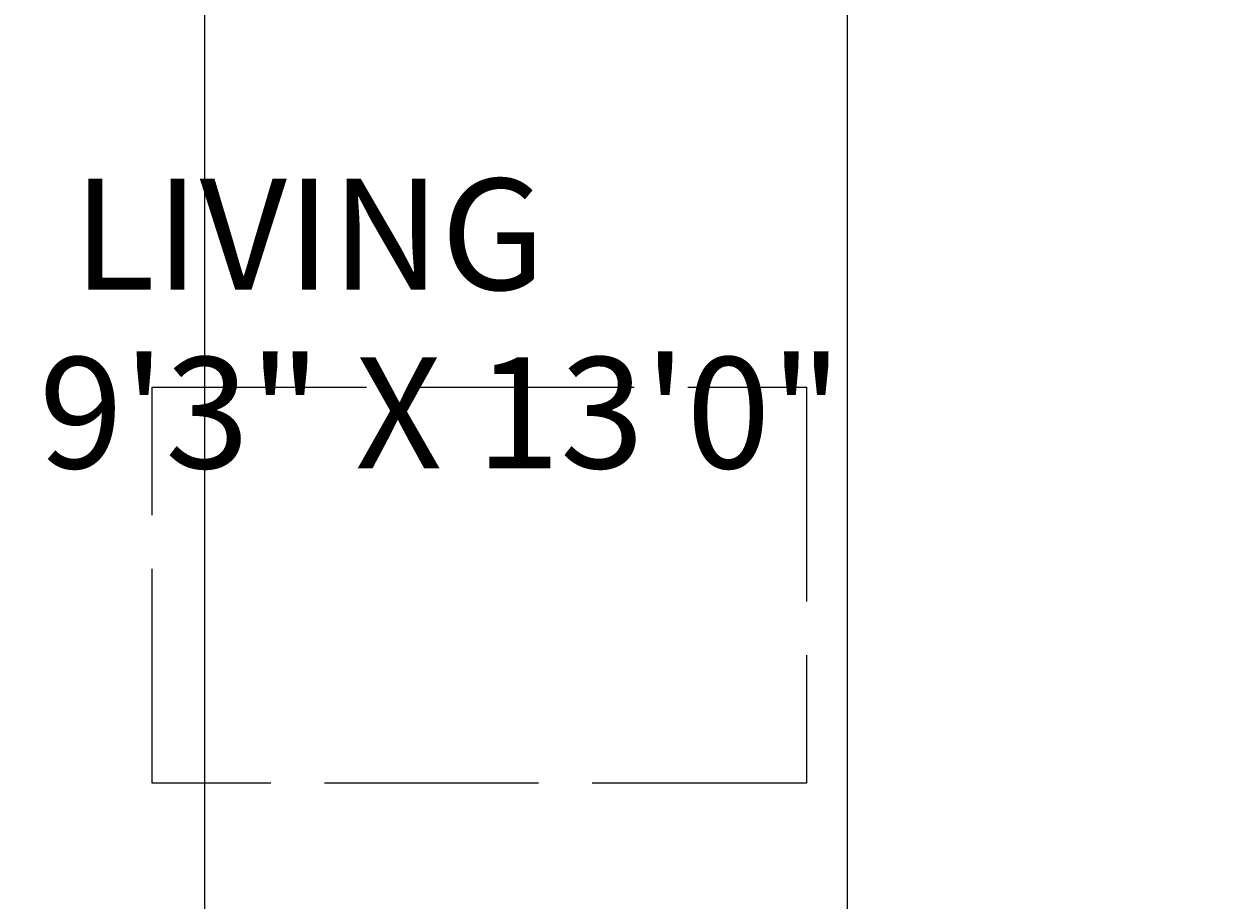
# Model space of a CAD drawing. Units: inches. Extents: x -61 to 1599, y -1316 to 257.
# Tile 110 of 204: x 170 to 236, y -117 to -68. Entities that reach past the tile are written whole.
import ezdxf

# ---------------------------------------------------------------- set-up
doc = ezdxf.new("R2010")
doc.units = ezdxf.units.IN
doc.header["$MEASUREMENT"] = 0
doc.linetypes.add('ACAD_ISO02W100', pattern=[15, 12, -3])
for name, color, linetype, lineweight in [('A-ANNO-DIMS', 2, 'Continuous', 18), ('A-AREA-IDEN', 1, 'Continuous', 18), ('A-FURN-LOW', 83, 'ACAD_ISO02W100', 18)]:
    doc.layers.add(name, color=color, linetype=linetype, lineweight=lineweight)
doc.styles.get("Standard").update_dxf_attribs({"font": 'arial.ttf'})
doc.dimstyles.get("Standard").update_dxf_attribs({"dimtxt": 0.18, "dimasz": 0.18, "dimexe": 0.18, "dimexo": 0.0625, "dimgap": 0.09, "dimtad": 0, "dimtih": 1, "dimtoh": 1, "dimdec": 0, "dimzin": 0, "dimdsep": 46, "dimlunit": 3, "dimtxsty": 'Standard', "dimcen": 0.09, "dimadec": 0, "dimazin": 0, "dimtfac": 1, "dimtdec": 0, "dimtofl": 0, "dimtmove": 0, "dimatfit": 3, "dimfxl": 1, "dimtolj": 1, "dimtzin": 0, "dimarcsym": 0})

# ---------------------------------------------------------------- blocks, each defined once
blk = doc.blocks.new('*D687')
at = {"layer": 'A-ANNO-DIMS', "color": 0, "lineweight": -2, "transparency": 16777216}
for p, q in [((289.418, 181.677), (-61.077, 181.677)), ((-60.897, 181.497), (-60.897, -528.952)), ((-60.897, -1239.765), (-60.897, -529.316)), ((319.64, -1239.945), (-61.077, -1239.945))]:
    blk.add_line(p, q, dxfattribs=at)
at = {"layer": 'A-ANNO-DIMS', "color": 0, "transparency": 16777216}
for points in [[(-60.927, 181.497), (-60.867, 181.497), (-60.897, 181.677)], [(-60.927, -1239.765), (-60.867, -1239.765), (-60.897, -1239.945)]]:
    blk.add_solid(points, dxfattribs=at)
at = {"layer": 'DEFPOINTS', "color": 0, "transparency": 16777216}
for p in [(289.481, 181.677), (-60.897, -1239.945), (319.703, -1239.945)]:
    blk.add_point(p, dxfattribs=at)
at = {"layer": 'A-ANNO-DIMS', "color": 0, "transparency": 16777216, "insert": (-60.897, -529.134), "char_height": 0.18, "attachment_point": 5}
blk.add_mtext('\\A1;1421.6', dxfattribs=at)
blk = doc.blocks.new('*D700')
at = {"layer": 'A-ANNO-DIMS', "color": 0, "lineweight": -2, "transparency": 16777216}
for p, q in [((14.703, -616.882), (14.703, 257.457)), ((14.883, 257.277), (96.772, 257.277)), ((179.572, 257.277), (97.683, 257.277)), ((179.752, -616.882), (179.752, 257.457))]:
    blk.add_line(p, q, dxfattribs=at)
at = {"layer": 'A-ANNO-DIMS', "color": 0, "transparency": 16777216}
for points in [[(14.883, 257.307), (14.883, 257.247), (14.703, 257.277)], [(179.572, 257.307), (179.572, 257.247), (179.752, 257.277)]]:
    blk.add_solid(points, dxfattribs=at)
at = {"layer": 'DEFPOINTS', "color": 0, "transparency": 16777216}
for p in [(179.752, 257.277), (14.703, -616.945), (179.752, -616.945)]:
    blk.add_point(p, dxfattribs=at)
at = {"layer": 'A-ANNO-DIMS', "color": 0, "transparency": 16777216, "insert": (97.227, 257.277), "char_height": 0.18, "attachment_point": 5}
blk.add_mtext('\\A1;165.05', dxfattribs=at)
blk = doc.blocks.new('*D701')
at = {"layer": 'A-ANNO-DIMS', "color": 0, "lineweight": -2, "transparency": 16777216}
for p, q in [((215.752, -616.882), (215.752, 257.457)), ((215.932, 257.277), (233.924, 257.277)), ((252.702, 257.277), (234.711, 257.277)), ((252.882, -616.882), (252.882, 257.457))]:
    blk.add_line(p, q, dxfattribs=at)
at = {"layer": 'A-ANNO-DIMS', "color": 0, "transparency": 16777216}
for points in [[(215.932, 257.307), (215.932, 257.247), (215.752, 257.277)], [(252.702, 257.307), (252.702, 257.247), (252.882, 257.277)]]:
    blk.add_solid(points, dxfattribs=at)
at = {"layer": 'DEFPOINTS', "color": 0, "transparency": 16777216}
for p in [(252.882, 257.277), (215.752, -616.945), (252.882, -616.945)]:
    blk.add_point(p, dxfattribs=at)
at = {"layer": 'A-ANNO-DIMS', "color": 0, "transparency": 16777216, "insert": (234.317, 257.277), "char_height": 0.18, "attachment_point": 5}
blk.add_mtext('\\A1;37.13', dxfattribs=at)

msp = doc.modelspace()

# ---------------------------------------------------------------- linework, layer by layer
at = {"layer": 'A-FURN-LOW'}
msp.add_lwpolyline([(213.4399, -110.6584), (176.794, -110.6584), (176.794, -88.492), (213.4399, -88.492)], close=True, dxfattribs=at)

# ---------------------------------------------------------------- texts
at = {"layer": 'A-AREA-IDEN'}
for s, height, p in [('   LIVING', 6.22364, (166.6485, -83.0336)), ('  9\'3" X 13\'0"', 6.223643, (166.6485, -93.0314))]:
    msp.add_text(s, height=height, dxfattribs=at).set_placement(p)

# ---------------------------------------------------------------- dimensions: what is measured, and where the dimension line sits
at = {"layer": 'A-ANNO-DIMS'}
for base, p1, p2, picture, middle in [((179.7521, 257.2771), (14.7028, -616.9446), (179.7521, -616.9446), '*D700', (97.2274, 257.2771)), ((252.8825, 257.2771), (215.7521, -616.9446), (252.8825, -616.9446), '*D701', (234.3173, 257.2771))]:
    dim = msp.add_linear_dim(base=base, p1=p1, p2=p2, dimstyle='Standard', override={"dimdec": 2, "dimlfac": 1, "dimrnd": 0, "dimzin": 0, "dimdsep": 46, "dimlunit": 2}, dxfattribs=at)
    dim.commit()
    dim.dimension.update_dxf_attribs({"geometry": picture, "text_midpoint": middle})
dim = msp.add_linear_dim(base=(-60.8972, -1239.9446), p1=(289.4807, 181.6771), p2=(319.7028, -1239.9446), angle=90, dimstyle='Standard', override={"dimdec": 1, "dimlfac": 1, "dimrnd": 0, "dimzin": 0, "dimdsep": 46, "dimlunit": 2}, dxfattribs=at)
dim.commit()
dim.dimension.update_dxf_attribs({"geometry": '*D687', "text_midpoint": (-60.8972, -529.1337)})

doc.saveas('drawing.dxf')
